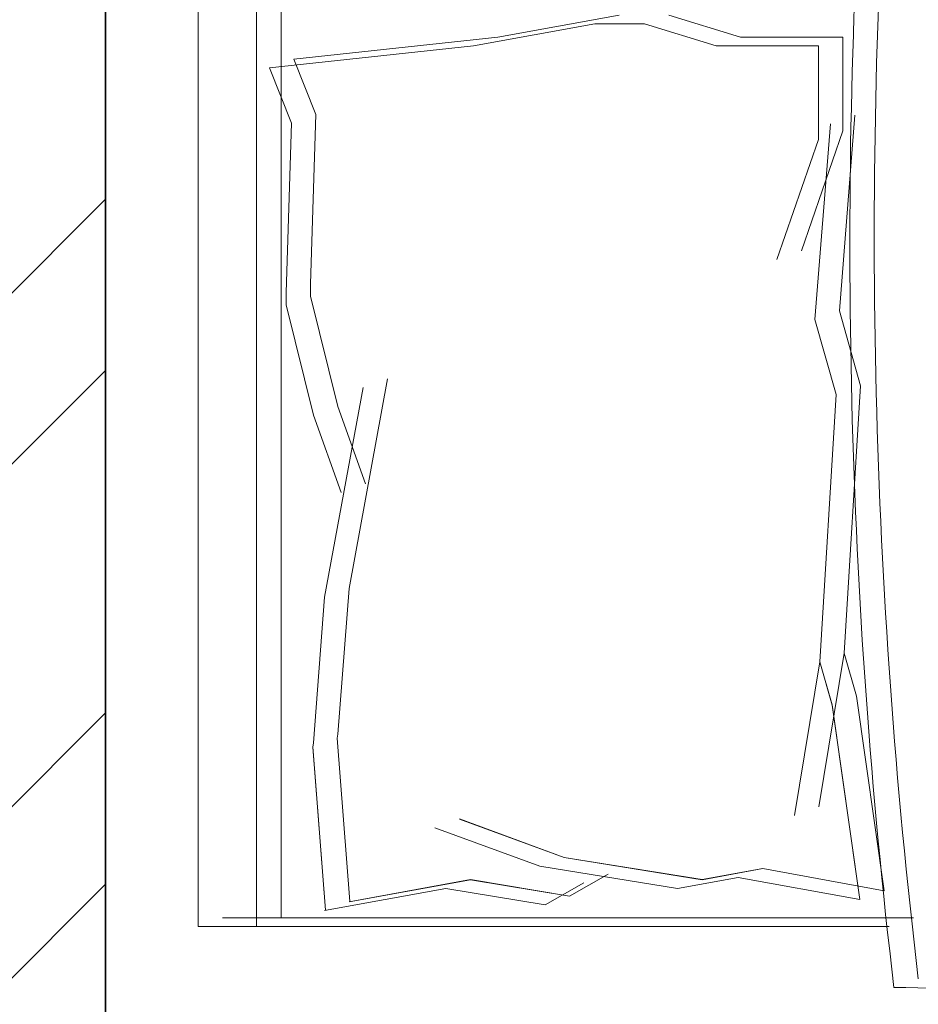
# Model space of a CAD drawing. Units: inches. Extents: x 2168 to 3056, y 1130 to 2629.
# Tile 25 of 42: x 2462 to 2485, y 2321 to 2347. Entities that reach past the tile are written whole.
import ezdxf

# ---------------------------------------------------------------- set-up
doc = ezdxf.new("R2010")
doc.units = ezdxf.units.IN
doc.layers.add('A-FURN', color=8, linetype='Continuous', lineweight=13)
doc.layers.add('A-WALL', color=7, linetype='Continuous', lineweight=35)
doc.layers.add('A-WALL-PATT', color=143, linetype='Continuous', lineweight=13, true_color=0x7aafdf)

# ---------------------------------------------------------------- blocks, each defined once
blk = doc.blocks.new('BED-DOUBLE')
for p, q in [((0, 3.475), (0, 51.494)), ((2.173, 3.704), (2.173, 51.494)), ((2.173, 3.703), (2.173, 51.494)), ((1.534, 3.475), (1.534, 51.266)), ((1.534, 3.475), (1.534, 51.265)), ((7.86, 26.789), (11.04, 27.368)), ((7.86, 26.789), (11.04, 27.367)), ((12.342, 27.368), (14.221, 26.789)), ((12.342, 27.367), (14.221, 26.789)), ((7.22, 26.561), (10.401, 27.139)), ((7.22, 26.561), (10.401, 27.139)), ((10.401, 27.139), (11.702, 27.139)), ((10.401, 27.139), (11.702, 27.139)), ((11.702, 27.139), (13.582, 26.561)), ((11.702, 27.139), (13.582, 26.561)), ((2.51, 26.211), (7.86, 26.789)), ((2.51, 26.211), (7.86, 26.789)), ((14.221, 26.789), (16.903, 26.789)), ((14.221, 26.789), (16.903, 26.789)), ((16.903, 26.789), (16.903, 24.332)), ((16.903, 26.789), (16.903, 24.332)), ((1.87, 25.983), (7.22, 26.561)), ((1.87, 25.983), (7.22, 26.561)), ((13.582, 26.561), (16.263, 26.561)), ((13.582, 26.561), (16.263, 26.561)), ((16.263, 26.561), (16.263, 24.104)), ((16.263, 26.561), (16.263, 24.103)), ((3.088, 24.766), (2.51, 26.211)), ((3.088, 24.765), (2.51, 26.211)), ((2.449, 24.537), (1.87, 25.983)), ((2.449, 24.537), (1.87, 25.983)), ((2.304, 20.092), (2.449, 24.537)), ((2.304, 20.091), (2.449, 24.537)), ((2.944, 20.32), (3.088, 24.766)), ((2.944, 20.32), (3.088, 24.765)), ((16.809, 19.613), (17.212, 24.744)), ((16.809, 19.612), (17.212, 24.744)), ((16.903, 24.332), (15.812, 21.187)), ((16.903, 24.332), (15.812, 21.187)), ((16.169, 19.384), (16.573, 24.516)), ((16.169, 19.384), (16.573, 24.516)), ((16.263, 24.104), (15.173, 20.959)), ((16.263, 24.103), (15.173, 20.959)), ((2.944, 19.998), (2.944, 20.32)), ((2.944, 19.998), (2.944, 20.32)), ((2.304, 19.77), (2.304, 20.092)), ((2.304, 19.77), (2.304, 20.091)), ((3.666, 17.107), (2.944, 19.998)), ((3.666, 17.107), (2.944, 19.998)), ((3.027, 16.879), (2.304, 19.77)), ((3.027, 16.879), (2.304, 19.77)), ((16.727, 17.424), (16.169, 19.384)), ((16.727, 17.424), (16.169, 19.384)), ((17.366, 17.652), (16.809, 19.613)), ((17.366, 17.652), (16.809, 19.612)), ((3.956, 12.337), (4.968, 17.83)), ((3.956, 12.337), (4.968, 17.83)), ((3.316, 12.109), (4.328, 17.602)), ((3.316, 12.108), (4.328, 17.601)), ((16.935, 10.642), (17.366, 17.652)), ((16.935, 10.642), (17.366, 17.652)), ((16.295, 10.414), (16.727, 17.424)), ((16.295, 10.414), (16.727, 17.424)), ((4.389, 15.083), (3.666, 17.107)), ((4.389, 15.083), (3.666, 17.107)), ((3.75, 14.855), (3.027, 16.879)), ((3.75, 14.855), (3.027, 16.879)), ((3.666, 8.513), (3.956, 12.337)), ((3.666, 8.513), (3.956, 12.337)), ((3.027, 8.285), (3.316, 12.109)), ((3.027, 8.285), (3.316, 12.108)), ((16.268, 6.61), (16.935, 10.642)), ((16.268, 6.61), (16.935, 10.642)), ((16.935, 10.642), (17.258, 9.509)), ((16.935, 10.642), (17.258, 9.509)), ((15.629, 6.382), (16.295, 10.414)), ((15.629, 6.382), (16.295, 10.414)), ((16.295, 10.414), (16.618, 9.281)), ((16.295, 10.414), (16.618, 9.28)), ((17.258, 9.509), (17.981, 4.412)), ((17.258, 9.509), (17.981, 4.412)), ((16.618, 9.281), (17.341, 4.184)), ((16.618, 9.28), (17.341, 4.184)), ((3.009, 8.18), (3.027, 8.285)), ((3.009, 8.179), (3.027, 8.285)), ((3.648, 8.408), (3.666, 8.513)), ((3.648, 8.408), (3.666, 8.513)), ((3.978, 4.127), (3.648, 8.408)), ((3.978, 4.127), (3.648, 8.408)), ((3.338, 3.899), (3.009, 8.18)), ((3.338, 3.899), (3.009, 8.179)), ((9.595, 5.28), (6.847, 6.292)), ((9.595, 5.279), (6.847, 6.291)), ((8.955, 5.051), (6.208, 6.063)), ((8.955, 5.051), (6.208, 6.063)), ((13.209, 4.702), (9.595, 5.28)), ((13.209, 4.701), (9.595, 5.279)), ((12.57, 4.473), (8.955, 5.051)), ((12.57, 4.473), (8.955, 5.051)), ((14.8, 4.991), (13.209, 4.702)), ((14.8, 4.99), (13.209, 4.701)), ((17.981, 4.412), (14.8, 4.991)), ((17.981, 4.412), (14.8, 4.99)), ((3.956, 4.123), (7.137, 4.702)), ((3.956, 4.123), (7.137, 4.701)), ((7.137, 4.702), (9.739, 4.268)), ((7.137, 4.701), (9.739, 4.268)), ((9.739, 4.268), (10.751, 4.846)), ((9.739, 4.268), (10.751, 4.846)), ((14.16, 4.762), (12.57, 4.473)), ((14.16, 4.762), (12.57, 4.473)), ((17.341, 4.184), (14.16, 4.762)), ((17.341, 4.184), (14.16, 4.762)), ((3.316, 3.895), (6.497, 4.473)), ((3.316, 3.895), (6.497, 4.473)), ((6.497, 4.473), (9.1, 4.039)), ((6.497, 4.473), (9.1, 4.039)), ((9.1, 4.039), (10.112, 4.618)), ((9.1, 4.039), (10.112, 4.617)), ((18.75, 3.704), (0.64, 3.704)), ((18.75, 3.703), (0.64, 3.703)), ((18.111, 3.475), (0, 3.475)), ((18.111, 3.475), (0, 3.475))]:
    blk.add_line(p, q)
for centre, radius, start, end in [((182.692, 21.587), 164.969, 176.08655, 186.78213), ((182.692, 21.587), 164.969, 176.08655, 186.78213), ((182.053, 21.359), 164.969, 176.08655, 186.78213), ((182.053, 21.359), 164.969, 176.08655, 186.78213), ((20.097, 85.162), 83.306, 268.72178, 275.60397), ((20.097, 85.162), 83.306, 268.72178, 275.60397)]:
    blk.add_arc(centre, radius, start, end)

msp = doc.modelspace()

# ---------------------------------------------------------------- hatches: boundary and pattern name
at = {"layer": 'A-WALL-PATT'}
h = msp.add_hatch(dxfattribs=at)
h.set_pattern_fill('ANSI32', color=256)
h.paths.add_polyline_path([(2463.796, 2409.389), (2467.387, 2409.389), (2467.387, 2413.889), (2454.768, 2413.889), (2454.768, 2411.639), (2454.768, 2409.389), (2459.296, 2409.389), (2459.296, 2265.389), (2455.644, 2265.389), (2455.644, 2260.889), (2467.349, 2260.889), (2467.349, 2263.139), (2467.349, 2265.389), (2463.796, 2265.389)])
h.paths.add_polyline_path([(2431.596, 2413.889), (2409.647, 2413.889), (2409.647, 2409.389), (2431.596, 2409.389), (2431.596, 2411.639)])
h.paths.add_polyline_path([(2349.647, 2413.889), (2331.796, 2413.889), (2331.796, 2362.671), (2336.296, 2362.671), (2336.296, 2409.389), (2349.647, 2409.389), (2349.647, 2411.639)])
h.paths.add_polyline_path([(2634.149, 2411.639), (2634.149, 2413.889), (2562.293, 2413.889), (2562.293, 2409.389), (2595.796, 2409.389), (2595.796, 2280.309), (2595.826, 2280.309), (2595.826, 2265.389), (2499.91, 2265.389), (2499.91, 2260.889), (2550.796, 2260.889), (2550.796, 2117.308), (2555.296, 2117.308), (2555.296, 2168.08), (2571.93, 2168.08), (2571.93, 2176.889), (2559.796, 2176.889), (2559.796, 2256.389), (2640.796, 2256.389), (2640.796, 2176.889), (2626.428, 2176.889), (2626.428, 2168.08), (2645.296, 2168.08), (2645.296, 2116.637), (2649.796, 2116.637), (2649.796, 2260.889), (2691.251, 2260.889), (2691.251, 2263.139), (2691.251, 2265.389), (2670.655, 2265.389), (2670.655, 2265.365), (2600.296, 2265.365), (2600.296, 2280.258), (2600.296, 2409.389), (2634.149, 2409.389)])
h.paths.add_polyline_path([(2600.296, 2473.889), (2612.84, 2473.889), (2612.84, 2478.389), (2572.636, 2478.389), (2572.636, 2473.889), (2595.796, 2473.889), (2595.796, 2413.889), (2600.296, 2413.889)])
h.paths.add_polyline_path([(2535.796, 2473.889), (2548.636, 2473.889), (2548.636, 2478.389), (2531.396, 2478.389), (2531.396, 2413.889), (2521.6, 2413.889), (2521.6, 2409.389), (2539.239, 2409.389), (2539.239, 2411.639), (2539.239, 2413.889), (2535.796, 2413.889)])
h.paths.add_polyline_path([(2664.796, 2478.389), (2636.84, 2478.389), (2636.84, 2473.889), (2660.296, 2473.889), (2660.296, 2413.889), (2656.165, 2413.889), (2656.165, 2409.389), (2671.684, 2409.389), (2671.684, 2411.639), (2671.684, 2413.889), (2664.796, 2413.889)])
h.paths.add_polyline_path([(2705.942, 2413.889), (2695.684, 2413.889), (2695.684, 2409.389), (2705.942, 2409.389)])
h.paths.add_polyline_path([(2741.35, 2413.889), (2728.733, 2413.889), (2728.733, 2411.639), (2728.733, 2409.389), (2732.296, 2409.389), (2732.296, 2265.389), (2725.733, 2265.389), (2725.733, 2260.889), (2740.917, 2260.889), (2740.917, 2263.139), (2740.917, 2265.389), (2736.796, 2265.389), (2736.796, 2409.389), (2741.35, 2409.389)])
h.paths.add_polyline_path([(2785.655, 2413.889), (2764.546, 2413.889), (2764.486, 2409.389), (2785.655, 2409.389), (2785.655, 2411.639)])
h.paths.add_polyline_path([(2864.296, 2413.889), (2845.655, 2413.889), (2845.655, 2409.389), (2859.796, 2409.389), (2859.796, 2368.425), (2864.296, 2368.425)])
h.paths.add_polyline_path([(2864.296, 2308.425), (2862.046, 2308.425), (2859.796, 2308.425), (2859.796, 2265.389), (2774.483, 2265.389), (2774.483, 2263.139), (2774.483, 2260.889), (2781.796, 2260.889), (2781.796, 2226.654), (2786.296, 2226.654), (2786.296, 2260.889), (2859.796, 2260.889), (2859.796, 2241.352), (2864.296, 2241.352)])
h.paths.add_polyline_path([(2864.296, 2217.352), (2862.046, 2217.352), (2859.796, 2217.352), (2859.796, 2200.889), (2786.296, 2200.889), (2786.296, 2205.931), (2784.046, 2205.931), (2781.796, 2205.931), (2781.796, 2150.974), (2786.296, 2150.974), (2786.296, 2161.889), (2859.796, 2161.889), (2859.796, 2144.419), (2864.296, 2144.419)])
h.paths.add_polyline_path([(2859.796, 2196.389), (2859.796, 2166.389), (2786.296, 2166.389), (2786.296, 2196.389)], flags=16)
h.paths.add_polyline_path([(2864.296, 2108.419), (2862.046, 2108.419), (2859.796, 2108.419), (2859.796, 2080.889), (2786.296, 2080.889), (2786.296, 2111.993), (2781.796, 2111.993), (2781.796, 2080.889), (2649.796, 2080.889), (2649.796, 2086.036), (2647.546, 2086.036), (2645.296, 2086.036), (2645.296, 2071.739), (2649.796, 2071.739), (2649.796, 2076.389), (2781.796, 2076.389), (2781.796, 2041.792), (2786.296, 2041.792), (2786.296, 2076.389), (2859.796, 2076.389), (2859.796, 2058.577), (2864.296, 2058.577)])
h.paths.add_polyline_path([(2864.296, 2022.577), (2859.796, 2022.577), (2859.796, 1992.389), (2786.296, 1992.389), (2786.296, 1999.573), (2781.796, 1999.573), (2781.796, 1848.085), (2784.046, 1848.085), (2786.296, 1848.085), (2786.296, 1851.389), (2859.796, 1851.389), (2859.796, 1838.258), (2864.296, 1838.258)], flags=17)
h.paths.add_polyline_path([(2859.796, 1987.889), (2859.796, 1855.889), (2786.296, 1855.889), (2786.296, 1987.889)], flags=16)
h.paths.add_polyline_path([(2823.046, 1987.889), (2841.421, 1921.889), (2823.046, 1855.889)], flags=0)
h.paths.add_polyline_path([(2864.296, 1814.258), (2859.796, 1814.258), (2859.796, 1791.389), (2786.296, 1791.389), (2786.296, 1825.658), (2784.046, 1825.658), (2781.796, 1825.658), (2781.796, 1791.389), (2720.155, 1791.389), (2720.155, 1791.265), (2649.796, 1791.265), (2649.796, 1806.159), (2649.796, 2038.983), (2647.546, 2038.983), (2645.296, 2038.983), (2645.296, 1783.925), (2649.796, 1783.925), (2649.796, 1786.889), (2781.796, 1786.889), (2781.796, 1746.789), (2786.296, 1746.789), (2786.296, 1786.889), (2859.796, 1786.889), (2859.796, 1770.083), (2864.296, 1770.083)])
h.paths.add_polyline_path([(2864.296, 1734.083), (2862.046, 1734.083), (2859.796, 1734.083), (2859.796, 1705.889), (2786.296, 1705.889), (2786.296, 1714.166), (2781.796, 1714.166), (2781.796, 1660.527), (2786.296, 1660.527), (2786.296, 1666.889), (2859.796, 1666.889), (2859.796, 1648.342), (2864.296, 1648.342)])
h.paths.add_polyline_path([(2786.296, 1701.389), (2859.796, 1701.389), (2859.796, 1671.389), (2786.296, 1671.389)], flags=16)
h.paths.add_polyline_path([(2649.796, 1756.576), (2647.546, 1756.576), (2645.296, 1756.576), (2645.296, 1606.889), (2555.296, 1606.889), (2555.296, 1749.513), (2553.046, 1749.513), (2550.796, 1749.513), (2550.796, 1606.889), (2503.006, 1606.889), (2503.006, 1604.639), (2503.006, 1602.389), (2595.796, 1602.389), (2595.849, 1602.389), (2595.849, 1587.495), (2595.796, 1458.389), (2561.502, 1458.389), (2561.502, 1456.139), (2561.502, 1453.889), (2595.796, 1453.889), (2595.796, 1381.889), (2573.438, 1381.889), (2573.438, 1377.389), (2613.01, 1377.389), (2613.01, 1379.639), (2613.01, 1381.889), (2600.296, 1381.889), (2600.296, 1453.889), (2634.327, 1453.889), (2634.327, 1458.389), (2600.296, 1458.389), (2600.296, 1602.389), (2670.655, 1602.389), (2694.095, 1602.389), (2694.095, 1606.889), (2649.796, 1606.889)])
h.paths.add_polyline_path([(2736.796, 1602.389), (2741.562, 1602.389), (2741.562, 1606.889), (2726.203, 1606.889), (2726.203, 1604.639), (2726.203, 1602.389), (2732.296, 1602.389), (2732.296, 1458.389), (2727.899, 1458.389), (2727.899, 1453.889), (2740.821, 1453.889), (2740.821, 1456.139), (2740.821, 1458.389), (2736.796, 1458.389)])
h.paths.add_polyline_path([(2859.796, 1606.889), (2786.296, 1606.889), (2786.296, 1637.334), (2784.046, 1637.334), (2781.796, 1637.334), (2781.796, 1606.889), (2775.612, 1606.889), (2775.612, 1602.389), (2859.796, 1602.389)])
h.paths.add_polyline_path([(2864.296, 1624.342), (2862.046, 1624.342), (2859.796, 1624.342), (2859.796, 1570.39), (2864.296, 1570.39)])
h.paths.add_polyline_path([(2864.296, 1510.39), (2862.046, 1510.39), (2859.796, 1510.39), (2859.796, 1458.389), (2846.735, 1458.389), (2846.735, 1456.139), (2846.735, 1453.889), (2864.296, 1453.889)])
h.paths.add_polyline_path([(2786.735, 1458.389), (2765.444, 1458.389), (2765.444, 1453.889), (2786.735, 1453.889)])
h.paths.add_polyline_path([(2706.004, 1458.389), (2695.36, 1458.389), (2695.36, 1453.889), (2706.004, 1453.889), (2706.004, 1456.139)])
h.paths.add_polyline_path([(2671.36, 1456.139), (2671.36, 1458.389), (2655.986, 1458.389), (2655.986, 1456.139), (2655.986, 1453.889), (2660.296, 1453.889), (2660.296, 1381.889), (2637.01, 1381.889), (2637.01, 1377.389), (2664.796, 1377.389), (2664.796, 1453.889), (2671.36, 1453.889)], flags=17)
h.paths.add_polyline_path([(2539.829, 1458.389), (2520.237, 1458.389), (2520.237, 1453.889), (2531.296, 1453.889), (2531.296, 1377.389), (2546.449, 1377.389), (2546.449, 1379.639), (2546.449, 1381.889), (2535.796, 1381.889), (2535.796, 1453.889), (2539.829, 1453.889)], flags=17)
h.paths.add_polyline_path([(2496.237, 1458.389), (2489.13, 1458.389), (2489.13, 1453.889), (2496.237, 1453.889), (2496.237, 1456.139)])
h.paths.add_polyline_path([(2467.433, 1456.139), (2467.433, 1458.389), (2463.796, 1458.389), (2463.796, 1602.389), (2468.242, 1602.389), (2468.242, 1605.7), (2468.242, 1606.889), (2454.602, 1606.889), (2454.602, 1602.389), (2459.296, 1602.389), (2459.296, 1458.389), (2454.24, 1458.389), (2454.24, 1453.889), (2467.433, 1453.889)])
h.paths.add_polyline_path([(2431.601, 1456.139), (2431.601, 1458.389), (2411.386, 1458.389), (2411.386, 1453.889), (2431.601, 1453.889)])
h.paths.add_polyline_path([(2351.386, 1458.389), (2336.296, 1458.389), (2336.296, 1490.693), (2334.046, 1490.693), (2331.796, 1490.693), (2331.796, 1453.889), (2351.386, 1453.889), (2351.386, 1456.139)])
h.paths.add_polyline_path([(2336.296, 1629.705), (2331.796, 1629.705), (2331.796, 1552.317), (2336.296, 1552.317), (2336.296, 1602.389), (2406.655, 1602.389), (2423.472, 1602.389), (2423.472, 1606.889), (2418.796, 1606.889), (2418.796, 1643.678), (2416.546, 1643.678), (2414.296, 1643.678), (2414.296, 1606.889), (2336.296, 1606.889)])
h.paths.add_polyline_path([(2418.796, 1714.384), (2414.296, 1714.384), (2414.296, 1705.889), (2336.296, 1705.889), (2336.296, 1731.324), (2334.046, 1731.324), (2331.796, 1731.324), (2331.796, 1653.705), (2334.046, 1653.705), (2336.296, 1653.705), (2336.296, 1666.889), (2414.296, 1666.889), (2414.296, 1663.589), (2418.796, 1663.589)])
h.paths.add_polyline_path([(2336.296, 1701.389), (2414.296, 1701.389), (2414.296, 1671.389), (2336.296, 1671.389)], flags=16)
h.paths.add_polyline_path([(2555.296, 2040.059), (2550.796, 2040.059), (2550.796, 1791.389), (2550.561, 1791.205), (2480.202, 1791.205), (2418.796, 1791.389), (2418.796, 1825.448), (2416.546, 1825.448), (2414.296, 1825.448), (2414.296, 1791.389), (2336.296, 1791.389), (2336.296, 1806.409), (2331.796, 1806.409), (2331.796, 1767.324), (2336.296, 1767.324), (2336.296, 1786.889), (2414.296, 1786.889), (2414.296, 1745.457), (2418.796, 1745.457), (2418.796, 1786.889), (2550.796, 1786.889), (2550.796, 1783.011), (2555.296, 1783.011)])
h.paths.add_polyline_path([(2418.796, 1923.389), (2423.207, 1923.389), (2423.207, 1925.639), (2423.207, 1927.889), (2418.796, 1927.889), (2418.796, 2000.048), (2414.296, 2000.048), (2414.296, 1992.389), (2336.296, 1992.389), (2336.296, 1987.889), (2414.296, 1987.889), (2414.296, 1855.889), (2336.296, 1855.889), (2336.296, 1851.389), (2414.296, 1851.389), (2414.296, 1846.759), (2418.796, 1846.759)], flags=17)
h.paths.add_polyline_path([(2336.296, 2019.294), (2334.046, 2019.294), (2331.796, 2019.294), (2331.796, 1830.409), (2336.296, 1830.409)], flags=17)
h.paths.add_polyline_path([(2550.796, 1927.889), (2453.541, 1927.889), (2453.541, 1925.639), (2453.541, 1923.389), (2550.796, 1923.389)], flags=17)
h.paths.add_polyline_path([(2744.987, 1927.889), (2649.796, 1927.889), (2649.796, 1923.389), (2744.987, 1923.389), (2744.987, 1925.639)], flags=17)
h.paths.add_polyline_path([(2555.296, 2086.458), (2553.046, 2086.458), (2550.796, 2086.458), (2550.796, 2080.889), (2418.796, 2080.889), (2336.296, 2080.889), (2336.296, 2115.399), (2334.046, 2115.399), (2331.796, 2115.399), (2331.796, 2055.294), (2336.296, 2055.294), (2336.296, 2076.389), (2550.796, 2076.389), (2550.796, 2071.538), (2555.296, 2071.538)])
h.paths.add_polyline_path([(2418.796, 2121.389), (2414.296, 2121.389), (2414.296, 2080.889), (2418.796, 2080.889)])
h.paths.add_polyline_path([(2418.796, 2076.389), (2414.296, 2076.389), (2414.296, 2035.123), (2418.796, 2035.123)])
h.paths.add_polyline_path([(2422.868, 2263.139), (2422.868, 2265.389), (2406.655, 2265.389), (2406.655, 2265.359), (2336.296, 2265.359), (2336.296, 2280.252), (2336.296, 2302.671), (2334.046, 2302.671), (2331.796, 2302.671), (2331.796, 2246.853), (2336.296, 2246.853), (2336.296, 2260.889), (2414.296, 2260.889), (2414.296, 2223.996), (2418.796, 2223.996), (2418.796, 2260.889), (2422.868, 2260.889)])
h.paths.add_polyline_path([(2418.796, 2204.783), (2416.546, 2204.783), (2414.296, 2204.783), (2414.296, 2200.889), (2336.296, 2200.889), (2336.296, 2220.853), (2331.796, 2220.853), (2331.796, 2151.399), (2336.296, 2151.399), (2336.296, 2161.889), (2414.296, 2161.889), (2414.296, 2153.726), (2418.796, 2153.726)])
h.paths.add_polyline_path([(2414.296, 2196.389), (2414.296, 2166.389), (2336.296, 2166.389), (2336.296, 2196.389)], flags=16)
h.paths.add_polyline_path([(2375.296, 2181.389), (2336.296, 2166.389), (2336.296, 2196.389)], flags=0)
h.paths.add_polyline_path([(2809.595, 2172.34), (2838.804, 2172.34), (2838.804, 2190.997), (2809.595, 2190.997)], flags=8)
h.paths.add_polyline_path([(2849.75, 1919.585), (2849.75, 1952.672), (2831.093, 1952.672), (2831.093, 1919.585)], flags=8)
h.paths.add_polyline_path([(2808.875, 1901.967), (2808.875, 1937.85), (2790.149, 1937.85), (2790.149, 1901.967)], flags=8)
h.paths.add_polyline_path([(2806.285, 1671.896), (2835.493, 1671.896), (2835.493, 1690.553), (2806.285, 1690.553)], flags=8)
h.paths.add_polyline_path([(2353.186, 1676.549), (2382.395, 1676.549), (2382.395, 1695.207), (2353.186, 1695.207)], flags=8)
h.paths.add_polyline_path([(2360.083, 1832.308), (2389.241, 1832.308), (2389.241, 1850.966), (2360.083, 1850.966)], flags=25)
h.paths.add_polyline_path([(2354.822, 2167.823), (2384.031, 2167.823), (2384.031, 2186.481), (2354.822, 2186.481)], flags=8)

# ---------------------------------------------------------------- linework, layer by layer
at = {"layer": 'A-WALL'}
msp.add_line((2463.796, 2409.389), (2463.796, 2265.389), dxfattribs=at)

# ---------------------------------------------------------------- block references
at = {"layer": 'A-FURN'}
msp.add_blockref('BED-DOUBLE', (2466.223, 2320.021), dxfattribs=at)

doc.saveas('drawing.dxf')
